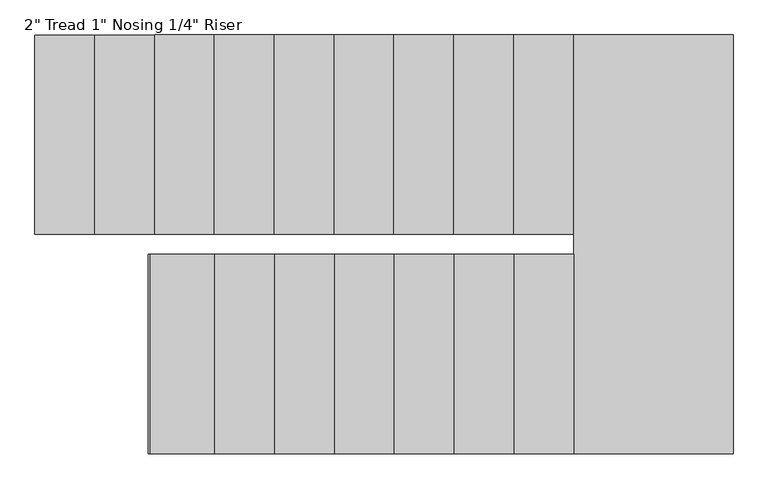
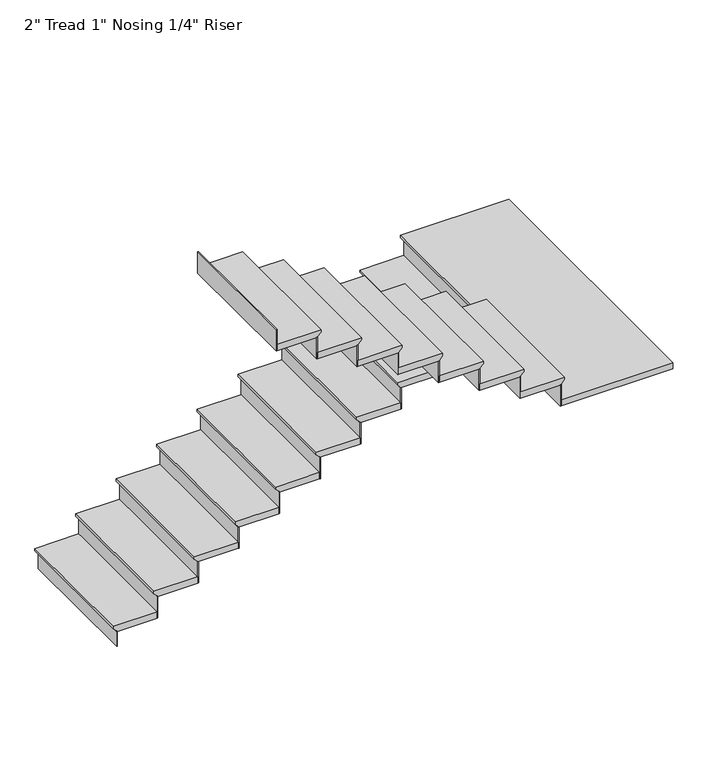
"""IFC4 building model written with IfcOpenShell, lengths in millimetres: stair flight geometry."""

from ifc_helpers import new_model, si_unit, origin, place, context, project, spatial, faceted_brep, source, transform, mapped, element, save


def stair_flight_68498a3f(model_context):
    return source(origin(), model_context, "Body", "Brep", [
        faceted_brep([(-12755.7436606, -2894.3024127, 455.0833333), (-12755.7436606, -2894.3024127, 474.1333333), (-12755.7436606, -1878.3024127, 474.1333333), (-12755.7436606, -1878.3024127, 455.0833333), (-12730.3436606, -2894.3024127, 429.6833333), (-12730.3436606, -1878.3024127, 429.6833333), (-12425.5436606, -2894.3024127, 474.1333333), (-12425.5436606, -1878.3024127, 474.1333333), (-12730.3436606, -1878.3024127, 423.3333333), (-12425.5436606, -1878.3024127, 423.3333333), (-12425.5436606, -2894.3024127, 423.3333333), (-12730.3436606, -2894.3024127, 423.3333333)], [[[0, 1, 2, 3]], [[4, 0, 3, 5]], [[2, 1, 6, 7]], [[8, 9, 10, 11]], [[2, 7, 9, 8, 5, 3]], [[8, 11, 4, 5]], [[6, 1, 0, 4, 11, 10]], [[7, 6, 10, 9]]]),
        faceted_brep([(-12730.3436606, -2894.3024127, 423.3333333), (-12730.3436606, -2894.3024127, 304.8), (-12723.9936606, -2894.3024127, 304.8), (-12723.9936606, -2894.3024127, 423.3333333), (-12730.3436606, -1878.3024127, 423.3333333), (-12723.9936606, -1878.3024127, 423.3333333), (-12723.9936606, -1878.3024127, 304.8), (-12730.3436606, -1878.3024127, 304.8)], [[[0, 1, 2, 3]], [[4, 5, 6, 7]], [[1, 0, 4, 7]], [[2, 1, 7, 6]], [[3, 2, 6, 5]], [[0, 3, 5, 4]]]),
        faceted_brep([(-12425.5436606, -2894.3024127, 592.6666667), (-12425.5436606, -2894.3024127, 423.3333333), (-12419.1936606, -2894.3024127, 423.3333333), (-12419.1936606, -2894.3024127, 592.6666667), (-12425.5436606, -1878.3024127, 592.6666667), (-12419.1936606, -1878.3024127, 592.6666667), (-12419.1936606, -1878.3024127, 423.3333333), (-12425.5436606, -1878.3024127, 423.3333333)], [[[0, 1, 2, 3]], [[4, 5, 6, 7]], [[1, 0, 4, 7]], [[2, 1, 7, 6]], [[3, 2, 6, 5]], [[0, 3, 5, 4]]]),
        faceted_brep([(-12450.9436606, -1878.3024127, 643.4666667), (-12450.9436606, -2894.3024127, 643.4666667), (-12120.7436606, -2894.3024127, 643.4666667), (-12120.7436606, -1878.3024127, 643.4666667), (-12425.5436606, -1878.3024127, 592.6666667), (-12120.7436606, -1878.3024127, 592.6666667), (-12120.7436606, -2894.3024127, 592.6666667), (-12425.5436606, -2894.3024127, 592.6666667), (-12425.5436606, -1878.3024127, 599.0166667), (-12450.9436606, -1878.3024127, 624.4166667), (-12425.5436606, -2894.3024127, 599.0166667), (-12450.9436606, -2894.3024127, 624.4166667)], [[[0, 1, 2, 3]], [[4, 5, 6, 7]], [[0, 3, 5, 4, 8, 9]], [[4, 7, 10, 8]], [[2, 1, 11, 10, 7, 6]], [[3, 2, 6, 5]], [[11, 1, 0, 9]], [[10, 11, 9, 8]]]),
        faceted_brep([(-12120.7436606, -2894.3024127, 762.0), (-12120.7436606, -2894.3024127, 592.6666667), (-12114.3936606, -2894.3024127, 592.6666667), (-12114.3936606, -2894.3024127, 762.0), (-12120.7436606, -1878.3024127, 762.0), (-12114.3936606, -1878.3024127, 762.0), (-12114.3936606, -1878.3024127, 592.6666667), (-12120.7436606, -1878.3024127, 592.6666667)], [[[0, 1, 2, 3]], [[4, 5, 6, 7]], [[1, 0, 4, 7]], [[2, 1, 7, 6]], [[3, 2, 6, 5]], [[0, 3, 5, 4]]]),
        faceted_brep([(-12146.1436606, -1878.3024127, 812.8), (-12146.1436606, -2894.3024127, 812.8), (-11815.9436606, -2894.3024127, 812.8), (-11815.9436606, -1878.3024127, 812.8), (-12120.7436606, -1878.3024127, 762.0), (-11815.9436606, -1878.3024127, 762.0), (-11815.9436606, -2894.3024127, 762.0), (-12120.7436606, -2894.3024127, 762.0), (-12120.7436606, -1878.3024127, 768.35), (-12146.1436606, -1878.3024127, 793.75), (-12120.7436606, -2894.3024127, 768.35), (-12146.1436606, -2894.3024127, 793.75)], [[[0, 1, 2, 3]], [[4, 5, 6, 7]], [[0, 3, 5, 4, 8, 9]], [[4, 7, 10, 8]], [[2, 1, 11, 10, 7, 6]], [[3, 2, 6, 5]], [[11, 1, 0, 9]], [[10, 11, 9, 8]]]),
        faceted_brep([(-11815.9436606, -2894.3024127, 931.3333333), (-11815.9436606, -2894.3024127, 762.0), (-11809.5936606, -2894.3024127, 762.0), (-11809.5936606, -2894.3024127, 931.3333333), (-11815.9436606, -1878.3024127, 931.3333333), (-11809.5936606, -1878.3024127, 931.3333333), (-11809.5936606, -1878.3024127, 762.0), (-11815.9436606, -1878.3024127, 762.0)], [[[0, 1, 2, 3]], [[4, 5, 6, 7]], [[1, 0, 4, 7]], [[2, 1, 7, 6]], [[3, 2, 6, 5]], [[0, 3, 5, 4]]]),
        faceted_brep([(-11841.3436606, -1878.3024127, 982.1333333), (-11841.3436606, -2894.3024127, 982.1333333), (-11511.1436606, -2894.3024127, 982.1333333), (-11511.1436606, -1878.3024127, 982.1333333), (-11815.9436606, -1878.3024127, 931.3333333), (-11511.1436606, -1878.3024127, 931.3333333), (-11511.1436606, -2894.3024127, 931.3333333), (-11815.9436606, -2894.3024127, 931.3333333), (-11815.9436606, -1878.3024127, 937.6833333), (-11841.3436606, -1878.3024127, 963.0833333), (-11815.9436606, -2894.3024127, 937.6833333), (-11841.3436606, -2894.3024127, 963.0833333)], [[[0, 1, 2, 3]], [[4, 5, 6, 7]], [[0, 3, 5, 4, 8, 9]], [[4, 7, 10, 8]], [[2, 1, 11, 10, 7, 6]], [[3, 2, 6, 5]], [[11, 1, 0, 9]], [[10, 11, 9, 8]]]),
        faceted_brep([(-11511.1436606, -2894.3024127, 1100.6666667), (-11511.1436606, -2894.3024127, 931.3333333), (-11504.7936606, -2894.3024127, 931.3333333), (-11504.7936606, -2894.3024127, 1100.6666667), (-11511.1436606, -1878.3024127, 1100.6666667), (-11504.7936606, -1878.3024127, 1100.6666667), (-11504.7936606, -1878.3024127, 931.3333333), (-11511.1436606, -1878.3024127, 931.3333333)], [[[0, 1, 2, 3]], [[4, 5, 6, 7]], [[1, 0, 4, 7]], [[2, 1, 7, 6]], [[3, 2, 6, 5]], [[0, 3, 5, 4]]]),
        faceted_brep([(-11536.5436606, -1878.3024127, 1151.4666667), (-11536.5436606, -2894.3024127, 1151.4666667), (-11206.3436606, -2894.3024127, 1151.4666667), (-11206.3436606, -1878.3024127, 1151.4666667), (-11511.1436606, -1878.3024127, 1100.6666667), (-11206.3436606, -1878.3024127, 1100.6666667), (-11206.3436606, -2894.3024127, 1100.6666667), (-11511.1436606, -2894.3024127, 1100.6666667), (-11511.1436606, -1878.3024127, 1107.0166667), (-11536.5436606, -1878.3024127, 1132.4166667), (-11511.1436606, -2894.3024127, 1107.0166667), (-11536.5436606, -2894.3024127, 1132.4166667)], [[[0, 1, 2, 3]], [[4, 5, 6, 7]], [[0, 3, 5, 4, 8, 9]], [[4, 7, 10, 8]], [[2, 1, 11, 10, 7, 6]], [[3, 2, 6, 5]], [[11, 1, 0, 9]], [[10, 11, 9, 8]]]),
        faceted_brep([(-11206.3436606, -2894.3024127, 1270.0), (-11206.3436606, -2894.3024127, 1100.6666667), (-11199.9936606, -2894.3024127, 1100.6666667), (-11199.9936606, -2894.3024127, 1270.0), (-11206.3436606, -1878.3024127, 1270.0), (-11199.9936606, -1878.3024127, 1270.0), (-11199.9936606, -1878.3024127, 1100.6666667), (-11206.3436606, -1878.3024127, 1100.6666667)], [[[0, 1, 2, 3]], [[4, 5, 6, 7]], [[1, 0, 4, 7]], [[2, 1, 7, 6]], [[3, 2, 6, 5]], [[0, 3, 5, 4]]]),
        faceted_brep([(-11231.7436606, -1878.3024127, 1320.8), (-11231.7436606, -2894.3024127, 1320.8), (-10901.5436606, -2894.3024127, 1320.8), (-10901.5436606, -1878.3024127, 1320.8), (-11206.3436606, -1878.3024127, 1270.0), (-10901.5436606, -1878.3024127, 1270.0), (-10901.5436606, -2894.3024127, 1270.0), (-11206.3436606, -2894.3024127, 1270.0), (-11206.3436606, -1878.3024127, 1276.35), (-11231.7436606, -1878.3024127, 1301.75), (-11206.3436606, -2894.3024127, 1276.35), (-11231.7436606, -2894.3024127, 1301.75)], [[[0, 1, 2, 3]], [[4, 5, 6, 7]], [[0, 3, 5, 4, 8, 9]], [[4, 7, 10, 8]], [[2, 1, 11, 10, 7, 6]], [[3, 2, 6, 5]], [[11, 1, 0, 9]], [[10, 11, 9, 8]]]),
        faceted_brep([(-10901.5436606, -2894.3024127, 1439.3333333), (-10901.5436606, -2894.3024127, 1270.0), (-10895.1936606, -2894.3024127, 1270.0), (-10895.1936606, -2894.3024127, 1439.3333333), (-10901.5436606, -1878.3024127, 1439.3333333), (-10895.1936606, -1878.3024127, 1439.3333333), (-10895.1936606, -1878.3024127, 1270.0), (-10901.5436606, -1878.3024127, 1270.0)], [[[0, 1, 2, 3]], [[4, 5, 6, 7]], [[1, 0, 4, 7]], [[2, 1, 7, 6]], [[3, 2, 6, 5]], [[0, 3, 5, 4]]]),
        faceted_brep([(-10926.9436606, -1878.3024127, 1490.1333333), (-10926.9436606, -2894.3024127, 1490.1333333), (-10596.7436606, -2894.3024127, 1490.1333333), (-10596.7436606, -1878.3024127, 1490.1333333), (-10901.5436606, -1878.3024127, 1439.3333333), (-10596.7436606, -1878.3024127, 1439.3333333), (-10596.7436606, -2894.3024127, 1439.3333333), (-10901.5436606, -2894.3024127, 1439.3333333), (-10901.5436606, -1878.3024127, 1445.6833333), (-10926.9436606, -1878.3024127, 1471.0833333), (-10901.5436606, -2894.3024127, 1445.6833333), (-10926.9436606, -2894.3024127, 1471.0833333)], [[[0, 1, 2, 3]], [[4, 5, 6, 7]], [[0, 3, 5, 4, 8, 9]], [[4, 7, 10, 8]], [[2, 1, 11, 10, 7, 6]], [[3, 2, 6, 5]], [[11, 1, 0, 9]], [[10, 11, 9, 8]]]),
        faceted_brep([(-10596.7436606, -2894.3024127, 1608.6666667), (-10596.7436606, -2894.3024127, 1439.3333333), (-10590.3936606, -2894.3024127, 1439.3333333), (-10590.3936606, -2894.3024127, 1608.6666667), (-10596.7436606, -1878.3024127, 1608.6666667), (-10590.3936606, -1878.3024127, 1608.6666667), (-10590.3936606, -1878.3024127, 1439.3333333), (-10596.7436606, -1878.3024127, 1439.3333333)], [[[0, 1, 2, 3]], [[4, 5, 6, 7]], [[1, 0, 4, 7]], [[2, 1, 7, 6]], [[3, 2, 6, 5]], [[0, 3, 5, 4]]]),
        faceted_brep([(-10622.1436606, -1878.3024127, 1659.4666667), (-10622.1436606, -2894.3024127, 1659.4666667), (-10291.9436606, -2894.3024127, 1659.4666667), (-10291.9436606, -1878.3024127, 1659.4666667), (-10596.7436606, -1878.3024127, 1608.6666667), (-10291.9436606, -1878.3024127, 1608.6666667), (-10291.9436606, -2894.3024127, 1608.6666667), (-10596.7436606, -2894.3024127, 1608.6666667), (-10596.7436606, -1878.3024127, 1615.0166667), (-10622.1436606, -1878.3024127, 1640.4166667), (-10596.7436606, -2894.3024127, 1615.0166667), (-10622.1436606, -2894.3024127, 1640.4166667)], [[[0, 1, 2, 3]], [[4, 5, 6, 7]], [[0, 3, 5, 4, 8, 9]], [[4, 7, 10, 8]], [[2, 1, 11, 10, 7, 6]], [[3, 2, 6, 5]], [[11, 1, 0, 9]], [[10, 11, 9, 8]]]),
        faceted_brep([(-10291.9436606, -2894.3024127, 1778.0), (-10291.9436606, -2894.3024127, 1608.6666667), (-10285.5936606, -2894.3024127, 1608.6666667), (-10285.5936606, -2894.3024127, 1778.0), (-10291.9436606, -1878.3024127, 1778.0), (-10285.5936606, -1878.3024127, 1778.0), (-10285.5936606, -1878.3024127, 1608.6666667), (-10291.9436606, -1878.3024127, 1608.6666667)], [[[0, 1, 2, 3]], [[4, 5, 6, 7]], [[1, 0, 4, 7]], [[2, 1, 7, 6]], [[3, 2, 6, 5]], [[0, 3, 5, 4]]]),
        faceted_brep([(-10317.3436606, -1878.3024127, 1828.8), (-10317.3436606, -2894.3024127, 1828.8), (-9987.1436606, -2894.3024127, 1828.8), (-9987.1436606, -1878.3024127, 1828.8), (-10291.9436606, -1878.3024127, 1778.0), (-9987.1436606, -1878.3024127, 1778.0), (-9987.1436606, -2894.3024127, 1778.0), (-10291.9436606, -2894.3024127, 1778.0), (-10291.9436606, -1878.3024127, 1784.35), (-10317.3436606, -1878.3024127, 1809.75), (-10291.9436606, -2894.3024127, 1784.35), (-10317.3436606, -2894.3024127, 1809.75)], [[[0, 1, 2, 3]], [[4, 5, 6, 7]], [[0, 3, 5, 4, 8, 9]], [[4, 7, 10, 8]], [[2, 1, 11, 10, 7, 6]], [[3, 2, 6, 5]], [[11, 1, 0, 9]], [[10, 11, 9, 8]]]),
        faceted_brep([(-9987.1436606, -2894.3024127, 1947.3333333), (-9987.1436606, -2894.3024127, 1778.0), (-9980.7936606, -2894.3024127, 1778.0), (-9980.7936606, -2894.3024127, 1947.3333333), (-9987.1436606, -1878.3024127, 1947.3333333), (-9980.7936606, -1878.3024127, 1947.3333333), (-9980.7936606, -1878.3024127, 1778.0), (-9987.1436606, -1878.3024127, 1778.0)], [[[0, 1, 2, 3]], [[4, 5, 6, 7]], [[1, 0, 4, 7]], [[2, 1, 7, 6]], [[3, 2, 6, 5]], [[0, 3, 5, 4]]]),
        faceted_brep([(-10037.9436606, -4011.9024127, 1998.1333333), (-9199.7436606, -4011.9024127, 1998.1333333), (-9199.7436606, -1878.3024127, 1998.1333333), (-10012.5436606, -1878.3024127, 1998.1333333), (-10012.5436606, -2995.9024127, 1998.1333333), (-10037.9436606, -2995.9024127, 1998.1333333), (-9199.7436606, -4011.9024127, 1947.3333333), (-10037.9436606, -4011.9024127, 1947.3333333), (-10037.9436606, -2995.9024127, 1947.3333333), (-10012.5436606, -2995.9024127, 1947.3333333), (-10012.5436606, -2894.3024127, 1947.3333333), (-9987.1436606, -2894.3024127, 1947.3333333), (-9987.1436606, -1878.3024127, 1947.3333333), (-9199.7436606, -1878.3024127, 1947.3333333), (-9987.1436606, -1878.3024127, 1953.6833333), (-10012.5436606, -1878.3024127, 1979.0833333), (-9987.1436606, -2894.3024127, 1953.6833333), (-10012.5436606, -2894.3024127, 1979.0833333)], [[[0, 1, 2, 3, 4, 5]], [[6, 7, 8, 9, 10, 11, 12, 13]], [[1, 0, 7, 6]], [[2, 1, 6, 13]], [[3, 2, 13, 12, 14, 15]], [[12, 11, 16, 14]], [[11, 10, 17, 16]], [[4, 3, 15, 17, 10, 9]], [[5, 4, 9, 8]], [[0, 5, 8, 7]], [[15, 14, 16, 17]]]),
        faceted_brep([(-10037.9436606, -2995.9024127, 2116.6666667), (-10037.9436606, -2995.9024127, 1947.3333333), (-10044.2936606, -2995.9024127, 1947.3333333), (-10044.2936606, -2995.9024127, 2116.6666667), (-10037.9436606, -4011.9024127, 2116.6666667), (-10044.2936606, -4011.9024127, 2116.6666667), (-10044.2936606, -4011.9024127, 1947.3333333), (-10037.9436606, -4011.9024127, 1947.3333333)], [[[0, 1, 2, 3]], [[4, 5, 6, 7]], [[1, 0, 4, 7]], [[2, 1, 7, 6]], [[3, 2, 6, 5]], [[0, 3, 5, 4]]]),
        faceted_brep([(-10012.5436606, -4011.9024127, 2167.4666667), (-10012.5436606, -2995.9024127, 2167.4666667), (-10342.7436606, -2995.9024127, 2167.4666667), (-10342.7436606, -4011.9024127, 2167.4666667), (-10037.9436606, -4011.9024127, 2116.6666667), (-10342.7436606, -4011.9024127, 2116.6666667), (-10342.7436606, -2995.9024127, 2116.6666667), (-10037.9436606, -2995.9024127, 2116.6666667), (-10037.9436606, -4011.9024127, 2123.0166667), (-10012.5436606, -4011.9024127, 2148.4166667), (-10037.9436606, -2995.9024127, 2123.0166667), (-10012.5436606, -2995.9024127, 2148.4166667)], [[[0, 1, 2, 3]], [[4, 5, 6, 7]], [[0, 3, 5, 4, 8, 9]], [[4, 7, 10, 8]], [[2, 1, 11, 10, 7, 6]], [[3, 2, 6, 5]], [[11, 1, 0, 9]], [[10, 11, 9, 8]]]),
        faceted_brep([(-10342.7436606, -2995.9024127, 2286.0), (-10342.7436606, -2995.9024127, 2116.6666667), (-10349.0936606, -2995.9024127, 2116.6666667), (-10349.0936606, -2995.9024127, 2286.0), (-10342.7436606, -4011.9024127, 2286.0), (-10349.0936606, -4011.9024127, 2286.0), (-10349.0936606, -4011.9024127, 2116.6666667), (-10342.7436606, -4011.9024127, 2116.6666667)], [[[0, 1, 2, 3]], [[4, 5, 6, 7]], [[1, 0, 4, 7]], [[2, 1, 7, 6]], [[3, 2, 6, 5]], [[0, 3, 5, 4]]]),
        faceted_brep([(-10317.3436606, -4011.9024127, 2336.8), (-10317.3436606, -2995.9024127, 2336.8), (-10647.5436606, -2995.9024127, 2336.8), (-10647.5436606, -4011.9024127, 2336.8), (-10342.7436606, -4011.9024127, 2286.0), (-10647.5436606, -4011.9024127, 2286.0), (-10647.5436606, -2995.9024127, 2286.0), (-10342.7436606, -2995.9024127, 2286.0), (-10342.7436606, -4011.9024127, 2292.35), (-10317.3436606, -4011.9024127, 2317.75), (-10342.7436606, -2995.9024127, 2292.35), (-10317.3436606, -2995.9024127, 2317.75)], [[[0, 1, 2, 3]], [[4, 5, 6, 7]], [[0, 3, 5, 4, 8, 9]], [[4, 7, 10, 8]], [[2, 1, 11, 10, 7, 6]], [[3, 2, 6, 5]], [[11, 1, 0, 9]], [[10, 11, 9, 8]]]),
        faceted_brep([(-10647.5436606, -2995.9024127, 2455.3333333), (-10647.5436606, -2995.9024127, 2286.0), (-10653.8936606, -2995.9024127, 2286.0), (-10653.8936606, -2995.9024127, 2455.3333333), (-10647.5436606, -4011.9024127, 2455.3333333), (-10653.8936606, -4011.9024127, 2455.3333333), (-10653.8936606, -4011.9024127, 2286.0), (-10647.5436606, -4011.9024127, 2286.0)], [[[0, 1, 2, 3]], [[4, 5, 6, 7]], [[1, 0, 4, 7]], [[2, 1, 7, 6]], [[3, 2, 6, 5]], [[0, 3, 5, 4]]]),
        faceted_brep([(-10622.1436606, -4011.9024127, 2506.1333333), (-10622.1436606, -2995.9024127, 2506.1333333), (-10952.3436606, -2995.9024127, 2506.1333333), (-10952.3436606, -4011.9024127, 2506.1333333), (-10647.5436606, -4011.9024127, 2455.3333333), (-10952.3436606, -4011.9024127, 2455.3333333), (-10952.3436606, -2995.9024127, 2455.3333333), (-10647.5436606, -2995.9024127, 2455.3333333), (-10647.5436606, -4011.9024127, 2461.6833333), (-10622.1436606, -4011.9024127, 2487.0833333), (-10647.5436606, -2995.9024127, 2461.6833333), (-10622.1436606, -2995.9024127, 2487.0833333)], [[[0, 1, 2, 3]], [[4, 5, 6, 7]], [[0, 3, 5, 4, 8, 9]], [[4, 7, 10, 8]], [[2, 1, 11, 10, 7, 6]], [[3, 2, 6, 5]], [[11, 1, 0, 9]], [[10, 11, 9, 8]]]),
        faceted_brep([(-10952.3436606, -2995.9024127, 2624.6666667), (-10952.3436606, -2995.9024127, 2455.3333333), (-10958.6936606, -2995.9024127, 2455.3333333), (-10958.6936606, -2995.9024127, 2624.6666667), (-10952.3436606, -4011.9024127, 2624.6666667), (-10958.6936606, -4011.9024127, 2624.6666667), (-10958.6936606, -4011.9024127, 2455.3333333), (-10952.3436606, -4011.9024127, 2455.3333333)], [[[0, 1, 2, 3]], [[4, 5, 6, 7]], [[1, 0, 4, 7]], [[2, 1, 7, 6]], [[3, 2, 6, 5]], [[0, 3, 5, 4]]]),
        faceted_brep([(-10926.9436606, -4011.9024127, 2675.4666667), (-10926.9436606, -2995.9024127, 2675.4666667), (-11257.1436606, -2995.9024127, 2675.4666667), (-11257.1436606, -4011.9024127, 2675.4666667), (-10952.3436606, -4011.9024127, 2624.6666667), (-11257.1436606, -4011.9024127, 2624.6666667), (-11257.1436606, -2995.9024127, 2624.6666667), (-10952.3436606, -2995.9024127, 2624.6666667), (-10952.3436606, -4011.9024127, 2631.0166667), (-10926.9436606, -4011.9024127, 2656.4166667), (-10952.3436606, -2995.9024127, 2631.0166667), (-10926.9436606, -2995.9024127, 2656.4166667)], [[[0, 1, 2, 3]], [[4, 5, 6, 7]], [[0, 3, 5, 4, 8, 9]], [[4, 7, 10, 8]], [[2, 1, 11, 10, 7, 6]], [[3, 2, 6, 5]], [[11, 1, 0, 9]], [[10, 11, 9, 8]]]),
        faceted_brep([(-11257.1436606, -2995.9024127, 2794.0), (-11257.1436606, -2995.9024127, 2624.6666667), (-11263.4936606, -2995.9024127, 2624.6666667), (-11263.4936606, -2995.9024127, 2794.0), (-11257.1436606, -4011.9024127, 2794.0), (-11263.4936606, -4011.9024127, 2794.0), (-11263.4936606, -4011.9024127, 2624.6666667), (-11257.1436606, -4011.9024127, 2624.6666667)], [[[0, 1, 2, 3]], [[4, 5, 6, 7]], [[1, 0, 4, 7]], [[2, 1, 7, 6]], [[3, 2, 6, 5]], [[0, 3, 5, 4]]]),
        faceted_brep([(-11231.7436606, -4011.9024127, 2844.8), (-11231.7436606, -2995.9024127, 2844.8), (-11561.9436606, -2995.9024127, 2844.8), (-11561.9436606, -4011.9024127, 2844.8), (-11257.1436606, -4011.9024127, 2794.0), (-11561.9436606, -4011.9024127, 2794.0), (-11561.9436606, -2995.9024127, 2794.0), (-11257.1436606, -2995.9024127, 2794.0), (-11257.1436606, -4011.9024127, 2800.35), (-11231.7436606, -4011.9024127, 2825.75), (-11257.1436606, -2995.9024127, 2800.35), (-11231.7436606, -2995.9024127, 2825.75)], [[[0, 1, 2, 3]], [[4, 5, 6, 7]], [[0, 3, 5, 4, 8, 9]], [[4, 7, 10, 8]], [[2, 1, 11, 10, 7, 6]], [[3, 2, 6, 5]], [[11, 1, 0, 9]], [[10, 11, 9, 8]]]),
        faceted_brep([(-11561.9436606, -2995.9024127, 2963.3333333), (-11561.9436606, -2995.9024127, 2794.0), (-11568.2936606, -2995.9024127, 2794.0), (-11568.2936606, -2995.9024127, 2963.3333333), (-11561.9436606, -4011.9024127, 2963.3333333), (-11568.2936606, -4011.9024127, 2963.3333333), (-11568.2936606, -4011.9024127, 2794.0), (-11561.9436606, -4011.9024127, 2794.0)], [[[0, 1, 2, 3]], [[4, 5, 6, 7]], [[1, 0, 4, 7]], [[2, 1, 7, 6]], [[3, 2, 6, 5]], [[0, 3, 5, 4]]]),
        faceted_brep([(-11536.5436606, -4011.9024127, 3014.1333333), (-11536.5436606, -2995.9024127, 3014.1333333), (-11866.7436606, -2995.9024127, 3014.1333333), (-11866.7436606, -4011.9024127, 3014.1333333), (-11561.9436606, -4011.9024127, 2963.3333333), (-11866.7436606, -4011.9024127, 2963.3333333), (-11866.7436606, -2995.9024127, 2963.3333333), (-11561.9436606, -2995.9024127, 2963.3333333), (-11561.9436606, -4011.9024127, 2969.6833333), (-11536.5436606, -4011.9024127, 2995.0833333), (-11561.9436606, -2995.9024127, 2969.6833333), (-11536.5436606, -2995.9024127, 2995.0833333)], [[[0, 1, 2, 3]], [[4, 5, 6, 7]], [[0, 3, 5, 4, 8, 9]], [[4, 7, 10, 8]], [[2, 1, 11, 10, 7, 6]], [[3, 2, 6, 5]], [[11, 1, 0, 9]], [[10, 11, 9, 8]]]),
        faceted_brep([(-11866.7436606, -2995.9024127, 3132.6666667), (-11866.7436606, -2995.9024127, 2963.3333333), (-11873.0936606, -2995.9024127, 2963.3333333), (-11873.0936606, -2995.9024127, 3132.6666667), (-11866.7436606, -4011.9024127, 3132.6666667), (-11873.0936606, -4011.9024127, 3132.6666667), (-11873.0936606, -4011.9024127, 2963.3333333), (-11866.7436606, -4011.9024127, 2963.3333333)], [[[0, 1, 2, 3]], [[4, 5, 6, 7]], [[1, 0, 4, 7]], [[2, 1, 7, 6]], [[3, 2, 6, 5]], [[0, 3, 5, 4]]]),
        faceted_brep([(-12171.5436606, -2995.9024127, 3302.0), (-12171.5436606, -2995.9024127, 3132.6666667), (-12177.8936606, -2995.9024127, 3132.6666667), (-12177.8936606, -2995.9024127, 3302.0), (-12171.5436606, -4011.9024127, 3302.0), (-12177.8936606, -4011.9024127, 3302.0), (-12177.8936606, -4011.9024127, 3132.6666667), (-12171.5436606, -4011.9024127, 3132.6666667)], [[[0, 1, 2, 3]], [[4, 5, 6, 7]], [[1, 0, 4, 7]], [[2, 1, 7, 6]], [[3, 2, 6, 5]], [[0, 3, 5, 4]]]),
        faceted_brep([(-11841.3436606, -4011.9024127, 3183.4666667), (-11841.3436606, -2995.9024127, 3183.4666667), (-12171.5436606, -2995.9024127, 3183.4666667), (-12171.5436606, -4011.9024127, 3183.4666667), (-11866.7436606, -4011.9024127, 3132.6666667), (-12171.5436606, -4011.9024127, 3132.6666667), (-12171.5436606, -2995.9024127, 3132.6666667), (-11866.7436606, -2995.9024127, 3132.6666667), (-11866.7436606, -4011.9024127, 3139.0166667), (-11841.3436606, -4011.9024127, 3164.4166667), (-11866.7436606, -2995.9024127, 3139.0166667), (-11841.3436606, -2995.9024127, 3164.4166667)], [[[0, 1, 2, 3]], [[4, 5, 6, 7]], [[0, 3, 5, 4, 8, 9]], [[4, 7, 10, 8]], [[2, 1, 11, 10, 7, 6]], [[3, 2, 6, 5]], [[11, 1, 0, 9]], [[10, 11, 9, 8]]]),
    ])


if __name__ == "__main__":
    model = new_model("IFC4")
    model_context = context("Model", 3, world=origin())
    ifc_project = project(units=[si_unit("LENGTHUNIT", "METRE", prefix="MILLI")], contexts=[model_context])
    site = spatial("IfcSite", under=ifc_project)
    building = spatial("IfcBuilding", under=site)
    placement = place(None, origin())
    stair_flight_shape = stair_flight_68498a3f(model_context)
    element("IfcStairFlight", 1, ObjectType="2\" Tread 1\" Nosing 1/4\" Riser", at=placement, inside=building, context=model_context, shape_type="MappedRepresentation", body=[
        mapped(stair_flight_shape, transform((0.0, 0.0, 0.0), x_axis=(1.0, 0.0, 0.0), y_axis=(0.0, 1.0, 0.0), z_axis=(0.0, 0.0, 1.0))),
    ])
    save(model, "model.ifc")

# Revit data of these elements
# Element 1 (IfcStairFlight, "2\" Tread 1\" Nosing 1/4\" Riser")
#   Materials on its faces: "Clad - White"
# Materials
#   "Clad - White": class "Wood", colour RGB 30 30 30, transparency 0, Cost = 0
